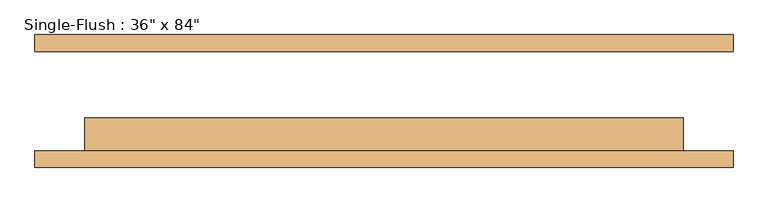
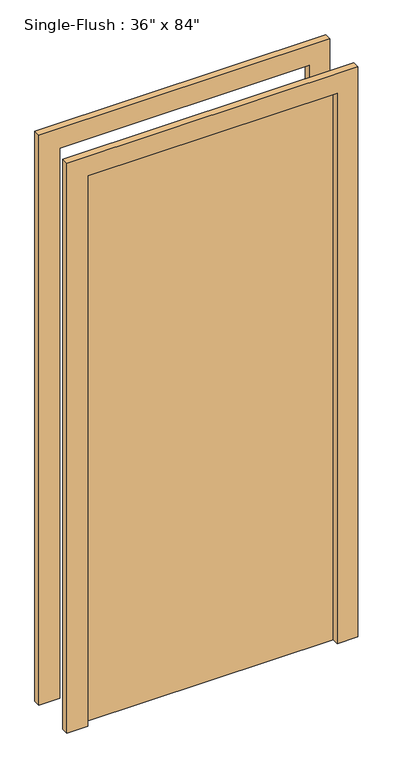
"""IFC4 building model written with IfcOpenShell, lengths in millimetres: door geometry."""

from ifc_helpers import new_model, si_unit, frame, origin, origin_with_axes, place, context, project, spatial, polyline, outline, extrude, source, transform, mapped, element, save


def door_686f89d2(model_context):
    return source(origin(), model_context, "Body", "SweptSolid", [
        extrude(outline(polyline([(2209.8, -533.4), (0.0, -533.4), (0.0, -457.2), (2133.6, -457.2), (2133.6, 457.2), (0.0, 457.2), (0.0, 533.4), (2209.8, 533.4), (2209.8, -533.4)])), frame((0.0, -101.6, 0.0), z_axis=(0.0, 1.0, 0.0), x_axis=(0.0, 0.0, 1.0)), (0.0, 0.0, 1.0), 25.4),
        extrude(outline(polyline([(2209.8, 533.4), (2209.8, -533.4), (0.0, -533.4), (0.0, -457.2), (2133.6, -457.2), (2133.6, 457.2), (0.0, 457.2), (0.0, 533.4), (2209.8, 533.4)])), frame((0.0, 76.2, 0.0), z_axis=(0.0, 1.0, 0.0), x_axis=(0.0, 0.0, 1.0)), (0.0, 0.0, 1.0), 25.4),
        extrude(outline(polyline([(457.2, -25.4), (457.2, -76.2), (-457.2, -76.2), (-457.2, -25.4), (457.2, -25.4)])), origin_with_axes(), (0.0, 0.0, 1.0), 2133.6),
    ])


if __name__ == "__main__":
    model = new_model("IFC4")
    model_context = context("Model", 3, world=origin())
    ifc_project = project(units=[si_unit("LENGTHUNIT", "METRE", prefix="MILLI")], contexts=[model_context])
    site = spatial("IfcSite", under=ifc_project)
    building = spatial("IfcBuilding", under=site)
    placement = place(None, origin())
    door_shape = door_686f89d2(model_context)
    element("IfcDoor", 1, ObjectType="Single-Flush : 36\" x 84\"", at=placement, inside=building, context=model_context, shape_type="MappedRepresentation", body=[
        mapped(door_shape, transform((0.0, 0.0, 0.0), x_axis=(1.0, 0.0, 0.0), y_axis=(0.0, 1.0, 0.0), z_axis=(0.0, 0.0, 1.0))),
    ])
    save(model, "model.ifc")

# Revit data of these elements
# Type "Single-Flush : 36\" x 84\""
#   Type Mark = "1"
#   Construction Type Id = "MDOOR"
#   Assembly Code = "C1020"
#   Analytic Construction = "Metal"
#   Thickness = 0' - 2"
#   Heat Transfer Coefficient (U) = 0.651978 BTU/(h·ft²·°F)
#   Height = 7' - 0"
#   Trim Projection Ext = 0' - 1"
#   Trim Projection Int = 0' - 1"
#   Trim Width = 0' - 3"
#   Width = 3' - 0"
#   Define Thermal Properties by = 1
#   Door Material = Door - Panel
#   Frame Material = Door - Frame
#   Visual Light Transmittance = 0
#   Solar Heat Gain Coefficient = 0
#   Function = (empty or 0)
#   Wall Closure = (empty or 0)
# Element 1 (IfcDoor, "Single-Flush : 36\" x 84\"")
#   Materials on its faces: "Door - Frame", "Door - Panel"
# Materials
#   "Door - Panel": class "Wood", colour RGB 210 159 95, transparency 0
#   "Door - Frame": colour RGB 118 70 51, transparency 0
